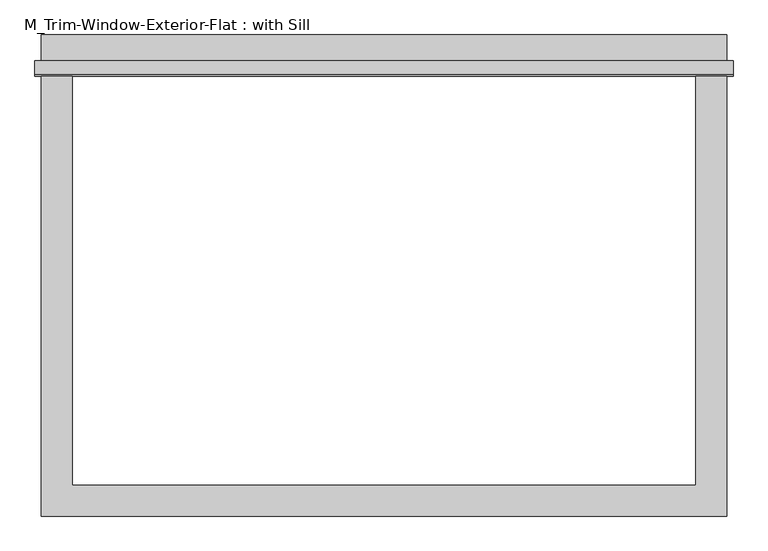
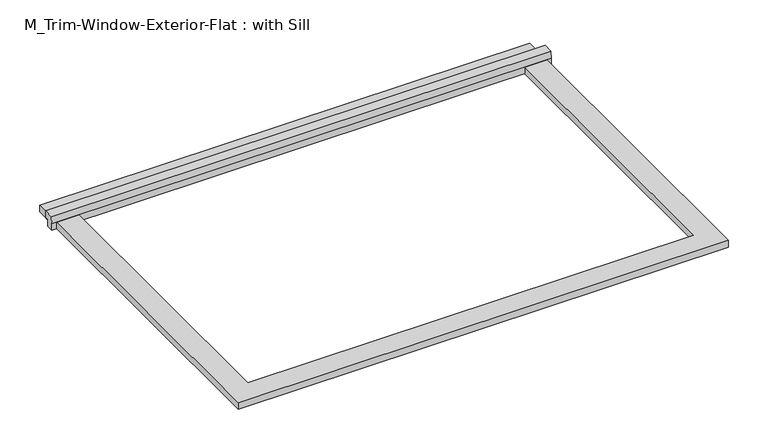
"""IFC4 building model written with IfcOpenShell, lengths in millimetres: proxy geometry, M_Trim-Window-Exterior-Flat : with Sill."""

from ifc_helpers import new_model, si_unit, frame, origin, origin_with_axes, place, context, project, spatial, polyline, outline, extrude, source, transform, mapped, element, save


def m_trim_window_exterior_flat_with_sill_1a4b2e7c(model_context):
    return source(origin(), model_context, "Body", "SweptSolid", [
        extrude(outline(polyline([(669.6, 820.4323709), (-669.6, 820.4323709), (-669.6, 880.4323709), (669.6, 880.4323709), (669.6, 820.4323709)])), origin_with_axes(), (0.0, 0.0, 1.0), 19.05),
        extrude(outline(polyline([(830.0, 38.1), (830.0, 19.05), (820.4323709, 19.05), (820.4323709, 0.0), (800.0, 0.0), (800.0, 19.05), (802.4580645, 38.1), (830.0, 38.1)])), frame((-682.3, 0.0, 0.0), z_axis=(1.0, 0.0, 0.0), x_axis=(0.0, 1.0, 0.0)), (0.0, 0.0, 1.0), 1364.6),
        extrude(outline(polyline([(-669.6, -60.0), (-669.6, 800.0), (-609.6, 800.0), (-609.6, 0.0), (609.6, 0.0), (609.6, 800.0), (669.6, 800.0), (669.6, -60.0), (-669.6, -60.0)])), origin_with_axes(), (0.0, 0.0, 1.0), 19.05),
    ])


if __name__ == "__main__":
    model = new_model("IFC4")
    model_context = context("Model", 3, world=origin())
    ifc_project = project(units=[si_unit("LENGTHUNIT", "METRE", prefix="MILLI")], contexts=[model_context])
    site = spatial("IfcSite", under=ifc_project)
    building = spatial("IfcBuilding", under=site)
    placement = place(None, origin())
    m_trim_window_exterior_flat_with_sill_shape = m_trim_window_exterior_flat_with_sill_1a4b2e7c(model_context)
    element("IfcBuildingElementProxy", 1, Name="M_Trim-Window-Exterior-Flat : with Sill", ObjectType="M_Trim-Window-Exterior-Flat : with Sill", at=placement, inside=building, context=model_context, shape_type="MappedRepresentation", body=[
        mapped(m_trim_window_exterior_flat_with_sill_shape, transform((0.0, 0.0, 0.0), x_axis=(1.0, 0.0, 0.0), y_axis=(0.0, 1.0, 0.0), z_axis=(0.0, 0.0, 1.0))),
    ])
    save(model, "model.ifc")

# Revit data of these elements
# Type "M_Trim-Window-Exterior-Flat : with Sill"
#   Trim Width = 0' - 2.3622"
#   Trim Thickness_Picture Frame = 0' - 1.1811"
#   Trim Thickness_with Sill = 0' - 0 3/4"
#   Sill Thickness = 0' - 1.1811"
#   Opening Width [instance default] = 1' - 11.62205"
#   Opening Height [instance default] = 2' - 11.43307"
#   Default Elevation = 3' - 11.24409"
#   Sill = yes
#   Picture Frame = no
#   Trim Material [instance default] = none
# Element 1 (IfcBuildingElementProxy, "M_Trim-Window-Exterior-Flat : with Sill")
#   Opening Width = 4' - 0"
#   Opening Height = 2' - 7.49606"
#   Trim Material = Clad - White
#   Materials on its faces: "Clad - White"
# Materials
#   "Clad - White": class "Wood", colour RGB 242 242 238, transparency 0, Cost = 0
